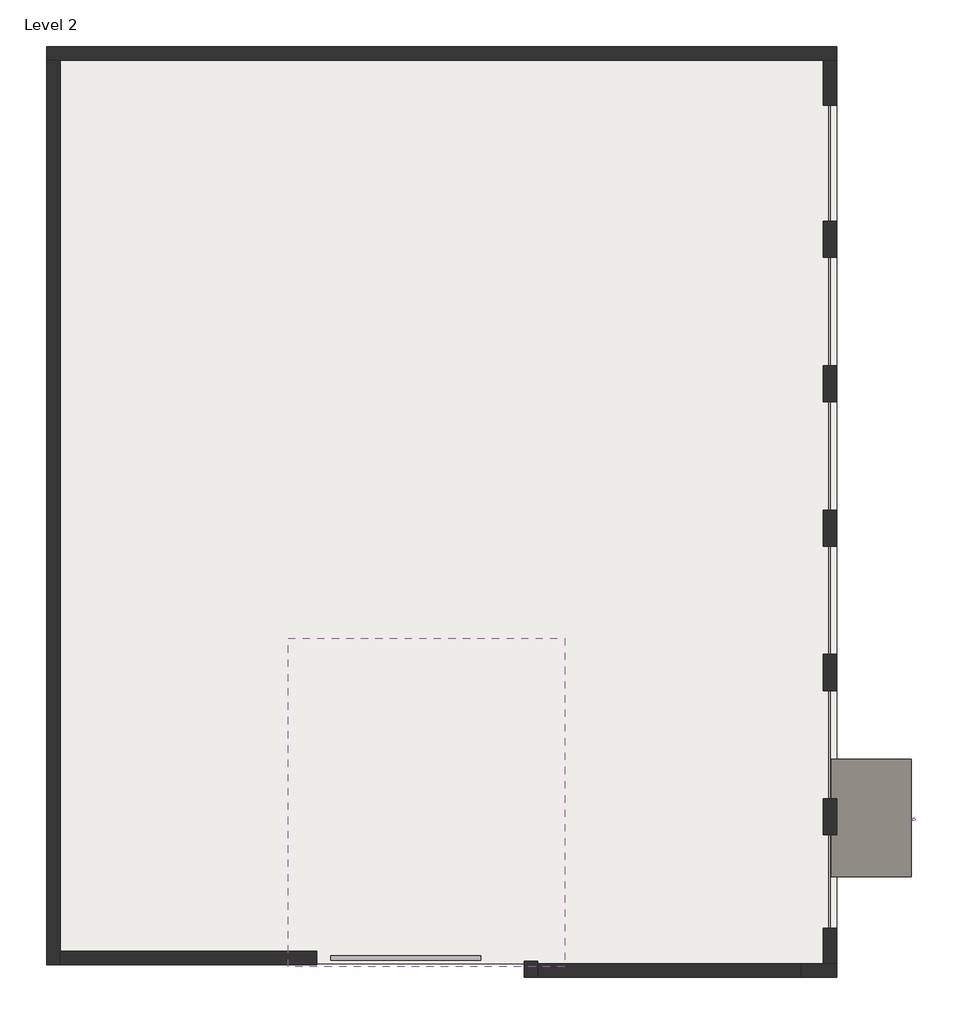
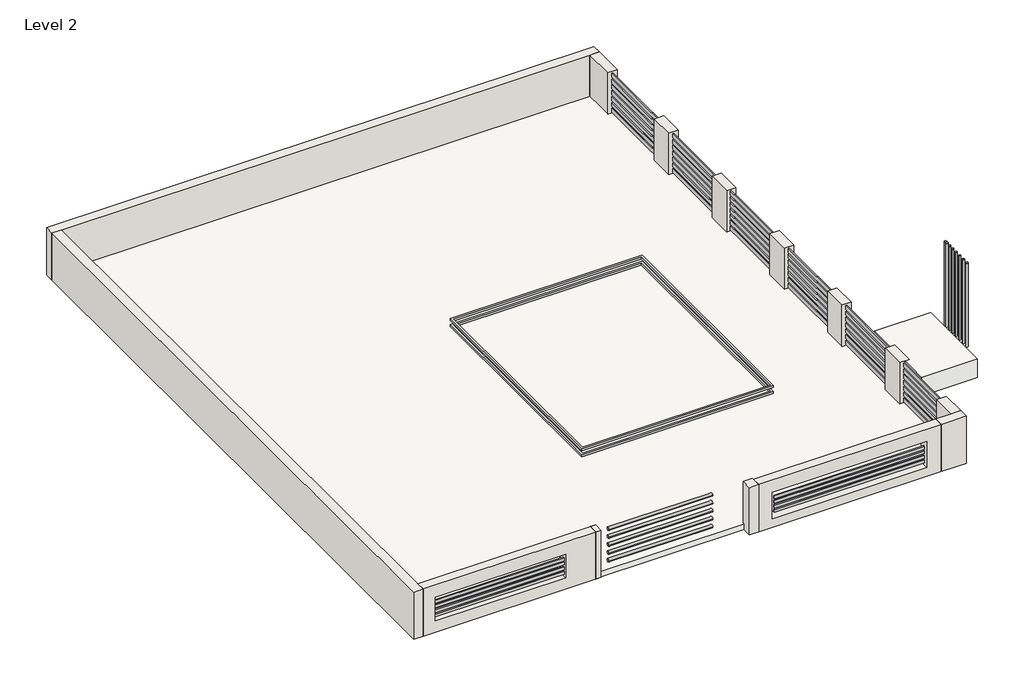
# One storey: 15 walls, 6 proxies, 1 covering, 1 slab.
"""IFC4 building model written with IfcOpenShell, lengths in millimetres."""

from ifc_helpers import new_model, si_unit, frame, origin, place, context, project, spatial, polyline, outline, extrude, faceted_brep, transform, mapped, element, save
from components import generic_models_12_generic_models_12_e0019dea, generic_models_2_generic_models_2_a69240e3, generic_models_3_generic_models_3_31b21ce6, generic_models_8_generic_models_8_cbadd6cc, railing_ms_1_railing_ms_1_2379e55e, railing_ms_2_railing_ms_1_4ed16cdf

model = new_model("IFC4")

# Units and contexts
model_context = context("Model", 3, world=origin())
ifc_project = project(units=[si_unit("LENGTHUNIT", "METRE", prefix="MILLI")], contexts=[model_context])

# Site, building, storey
site = spatial("IfcSite", under=ifc_project)
building = spatial("IfcBuilding", under=site)
storey = spatial("IfcBuildingStorey", under=building, Name="Level 2", Elevation=6705.6)

# Proxies
placement = place(None, origin())
generic_models_12_generic_models_12_shape = generic_models_12_generic_models_12_e0019dea(model_context)
element("IfcBuildingElementProxy", 1, Name="Generic Models 12 : Generic Models 12", ObjectType="Generic Models 12 : Generic Models 12", at=placement, inside=storey, context=model_context, shape_type="MappedRepresentation", body=[
    mapped(generic_models_12_generic_models_12_shape, transform((0.0, 0.0, 0.0), x_axis=(1.0, 0.0, 0.0), y_axis=(0.0, 1.0, 0.0), z_axis=(0.0, 0.0, 1.0))),
])
generic_models_2_generic_models_2_shape = generic_models_2_generic_models_2_a69240e3(model_context)
element("IfcBuildingElementProxy", 2, Name="Generic Models 2 : Generic Models 2", ObjectType="Generic Models 2 : Generic Models 2", at=placement, inside=storey, context=model_context, shape_type="MappedRepresentation", body=[
    mapped(generic_models_2_generic_models_2_shape, transform((0.0, 0.0, 0.0), x_axis=(1.0, 0.0, 0.0), y_axis=(0.0, 1.0, 0.0), z_axis=(0.0, 0.0, 1.0))),
])
generic_models_3_generic_models_3_shape = generic_models_3_generic_models_3_31b21ce6(model_context)
element("IfcBuildingElementProxy", 3, Name="Generic Models 3 : Generic Models 3", ObjectType="Generic Models 3 : Generic Models 3", at=placement, inside=storey, context=model_context, shape_type="MappedRepresentation", body=[
    mapped(generic_models_3_generic_models_3_shape, transform((0.0, 0.0, 0.0), x_axis=(1.0, 0.0, 0.0), y_axis=(0.0, 1.0, 0.0), z_axis=(0.0, 0.0, 1.0))),
])
generic_models_8_generic_models_8_shape = generic_models_8_generic_models_8_cbadd6cc(model_context)
element("IfcBuildingElementProxy", 4, Name="Generic Models 8 : Generic Models 8", ObjectType="Generic Models 8 : Generic Models 8", at=placement, inside=storey, context=model_context, shape_type="MappedRepresentation", body=[
    mapped(generic_models_8_generic_models_8_shape, transform((0.0, 0.0, 0.0), x_axis=(1.0, 0.0, 0.0), y_axis=(0.0, 1.0, 0.0), z_axis=(0.0, 0.0, 1.0))),
])
railing_ms_1_railing_ms_1_shape = railing_ms_1_railing_ms_1_2379e55e(model_context)
element("IfcBuildingElementProxy", 5, Name="railing ms 1 : railing ms 1", ObjectType="railing ms 1 : railing ms 1", at=placement, inside=storey, context=model_context, shape_type="MappedRepresentation", body=[
    mapped(railing_ms_1_railing_ms_1_shape, transform((0.0, 0.0, 0.0), x_axis=(1.0, 0.0, 0.0), y_axis=(0.0, 1.0, 0.0), z_axis=(0.0, 0.0, 1.0))),
])
railing_ms_2_railing_ms_1_shape = railing_ms_2_railing_ms_1_4ed16cdf(model_context)
element("IfcBuildingElementProxy", 6, Name="railing ms 2 : railing ms 1", ObjectType="railing ms 2 : railing ms 1", at=placement, inside=storey, context=model_context, shape_type="MappedRepresentation", body=[
    mapped(railing_ms_2_railing_ms_1_shape, transform((8178.1160753, -127.0, -19.7286522), x_axis=(1.0, 0.0, 0.0), y_axis=(0.0, 1.0, 0.0), z_axis=(0.0, 0.0, 1.0))),
])

# Covering
element("IfcCovering", 7, ObjectType="300mm_Generic 3", at=placement, inside=storey, context=model_context, shape_type="SweptSolid", body=[
    extrude(outline(polyline([(-19412.729089, -4479.5968048), (-19412.729089, 10900.1031952), (-6179.329089, 10900.1031952), (-6179.329089, -4593.8968048), (-6788.929089, -4593.8968048), (-11348.229089, -4593.8968048), (-11348.229089, -4479.5968048), (-19412.729089, -4479.5968048)])), frame((0.0, 0.0, 6705.6), z_axis=(0.0, 0.0, 1.0), x_axis=(1.0, 0.0, 0.0)), (0.0, 0.0, 1.0), 152.4),
])

# Slab
element("IfcSlab", 8, ObjectType="Floor-Grnd-Susp_65Scr-80Ins-100Blk-75PC", at=placement, inside=storey, context=model_context, shape_type="SweptSolid", body=[
    extrude(outline(polyline([(-4918.5966301, -1025.1968048), (-4918.5966301, -3006.3968048), (-6274.579089, -3006.3968048), (-6274.579089, -1025.1968048), (-4918.5966301, -1025.1968048)])), frame((0.0, 0.0, 7448.45), z_axis=(0.0, 0.0, 1.0), x_axis=(1.0, 0.0, 0.0)), (0.0, 0.0, 1.0), 470.0),
])

# Walls
element("IfcWall", 9, ObjectType="basic wall 2", at=placement, inside=storey, context=model_context, shape_type="Brep", body=[
    faceted_brep([(-6179.329089, 11014.4031952, 6705.6), (-19527.029089, 11014.4031952, 6705.6), (-19527.029089, 11014.4031952, 7924.8), (-6179.329089, 11014.4031952, 7924.8), (-6179.329089, 10785.8031952, 6705.6), (-6179.329089, 10785.8031952, 7924.8), (-6407.929089, 10785.8031952, 7924.8), (-19298.429089, 10785.8031952, 7924.8), (-19527.029089, 10785.8031952, 7924.8), (-19527.029089, 10785.8031952, 6705.6), (-19298.429089, 10785.8031952, 6705.6), (-6407.929089, 10785.8031952, 6705.6)], [[[0, 1, 2, 3]], [[4, 5, 6, 7, 8, 9, 10, 11]], [[1, 0, 4, 11, 10, 9]], [[3, 2, 8, 7, 6, 5]], [[2, 1, 9, 8]], [[0, 3, 5, 4]]]),
])
element("IfcWall", 10, ObjectType="basic wall 2", at=placement, inside=storey, context=model_context, shape_type="Brep", body=[
    faceted_brep([(-19527.029089, 10785.8031952, 6705.6), (-19527.029089, -4496.0724035, 6705.6), (-19527.029089, -4496.0724035, 7924.8), (-19527.029089, 10785.8031952, 7924.8), (-19298.429089, 10785.8031952, 6705.6), (-19298.429089, 10785.8031952, 7924.8), (-19298.429089, -4267.4724035, 7924.8), (-19298.429089, -4496.0724035, 7924.8), (-19298.429089, -4496.0724035, 6705.6), (-19298.429089, -4267.4724035, 6705.6)], [[[0, 1, 2, 3]], [[4, 5, 6, 7, 8, 9]], [[1, 0, 4, 9, 8]], [[3, 2, 7, 6, 5]], [[0, 3, 5, 4]], [[2, 1, 8, 7]]]),
])
element("IfcWall", 11, ObjectType="basic wall 2", at=placement, inside=storey, context=model_context, shape_type="SweptSolid", body=[
    extrude(outline(polyline([(6705.6, -19298.429089), (6705.6, -14961.379089), (7924.8, -14961.379089), (7924.8, -19298.429089), (6705.6, -19298.429089)]), holes=[polyline([(7605.6, -15821.923818), (6996.0, -15821.923818), (6996.0, -19004.329089), (7605.6, -19004.329089), (7605.6, -15821.923818)])]), frame((0.0, -4496.0724035, 0.0), z_axis=(0.0, 1.0, 0.0), x_axis=(0.0, 0.0, 1.0)), (0.0, 0.0, 1.0), 228.6),
])
element("IfcWall", 12, ObjectType="basic wall 2", at=placement, inside=storey, context=model_context, shape_type="SweptSolid", body=[
    extrude(outline(polyline([(6705.6, -11233.929089), (6705.6, -6788.929089), (7924.8, -6788.929089), (7924.8, -11233.929089), (6705.6, -11233.929089)]), holes=[polyline([(7605.6, -7141.2969384), (6930.6, -7141.2969384), (6930.6, -10904.329089), (7605.6, -10904.329089), (7605.6, -7141.2969384)])]), frame((0.0, -4708.1968048, 0.0), z_axis=(0.0, 1.0, 0.0), x_axis=(0.0, 0.0, 1.0)), (0.0, 0.0, 1.0), 228.6),
])
element("IfcWall", 13, ObjectType="basic wall 2", at=placement, inside=storey, context=model_context, shape_type="Brep", body=[
    faceted_brep([(-11233.929089, -4708.1968048, 6705.6), (-11233.929089, -4479.5968048, 6705.6), (-11233.929089, -4438.9224035, 6705.6), (-11233.929089, -4438.9224035, 7924.8), (-11233.929089, -4479.5968048, 7924.8), (-11233.929089, -4708.1968048, 7924.8), (-11462.529089, -4708.1968048, 6705.6), (-11462.529089, -4708.1968048, 7924.8), (-11462.529089, -4438.9224035, 7924.8), (-11462.529089, -4438.9224035, 6705.6)], [[[0, 1, 2, 3, 4, 5]], [[6, 7, 8, 9]], [[2, 1, 0, 6, 9]], [[5, 4, 3, 8, 7]], [[0, 5, 7, 6]], [[3, 2, 9, 8]]]),
])
element("IfcWall", 14, ObjectType="basic wall 2", at=placement, inside=storey, context=model_context, shape_type="Brep", body=[
    faceted_brep([(-6788.929089, -4708.1968048, 7924.8), (-6788.929089, -4708.1968048, 6705.6), (-6179.329089, -4708.1968048, 6705.6), (-6179.329089, -4708.1968048, 7924.8), (-6788.929089, -4479.5968048, 6705.6), (-6788.929089, -4479.5968048, 7924.8), (-6407.929089, -4479.5968048, 7924.8), (-6179.329089, -4479.5968048, 7924.8), (-6179.329089, -4479.5968048, 6705.6), (-6407.929089, -4479.5968048, 6705.6)], [[[0, 1, 2, 3]], [[4, 5, 6, 7, 8, 9]], [[2, 1, 4, 9, 8]], [[0, 3, 7, 6, 5]], [[0, 5, 4, 1]], [[3, 2, 8, 7]]]),
])
element("IfcWall", 15, ObjectType="basic wall 2", at=placement, inside=storey, context=model_context, shape_type="SweptSolid", body=[
    extrude(outline(polyline([(-15088.379089, -4267.4724035), (-14961.379089, -4267.4724035), (-14961.379089, -4496.0724035), (-15088.379089, -4496.0724035), (-15088.379089, -4267.4724035)])), frame((0.0, 0.0, 6705.6), z_axis=(0.0, 0.0, 1.0), x_axis=(1.0, 0.0, 0.0)), (0.0, 0.0, 1.0), 1219.2),
])
element("IfcWall", 16, ObjectType="basic wall 2", at=placement, inside=storey, context=model_context, shape_type="SweptSolid", body=[
    extrude(outline(polyline([(-6179.329089, -1691.9468048), (-6179.329089, -2301.5468048), (-6407.929089, -2301.5468048), (-6407.929089, -1691.9468048), (-6179.329089, -1691.9468048)])), frame((0.0, 0.0, 6705.6), z_axis=(0.0, 0.0, 1.0), x_axis=(1.0, 0.0, 0.0)), (0.0, 0.0, 1.0), 1219.2),
])
element("IfcWall", 17, ObjectType="basic wall 2", at=placement, inside=storey, context=model_context, shape_type="SweptSolid", body=[
    extrude(outline(polyline([(-6179.329089, 746.4531952), (-6179.329089, 136.8531952), (-6407.929089, 136.8531952), (-6407.929089, 746.4531952), (-6179.329089, 746.4531952)])), frame((0.0, 0.0, 6705.6), z_axis=(0.0, 0.0, 1.0), x_axis=(1.0, 0.0, 0.0)), (0.0, 0.0, 1.0), 1219.2),
])
element("IfcWall", 18, ObjectType="basic wall 2", at=placement, inside=storey, context=model_context, shape_type="SweptSolid", body=[
    extrude(outline(polyline([(-6179.329089, 3184.8531952), (-6179.329089, 2575.2531952), (-6407.929089, 2575.2531952), (-6407.929089, 3184.8531952), (-6179.329089, 3184.8531952)])), frame((0.0, 0.0, 6705.6), z_axis=(0.0, 0.0, 1.0), x_axis=(1.0, 0.0, 0.0)), (0.0, 0.0, 1.0), 1219.2),
])
element("IfcWall", 19, ObjectType="basic wall 2", at=placement, inside=storey, context=model_context, shape_type="SweptSolid", body=[
    extrude(outline(polyline([(-6179.329089, 5623.2531952), (-6179.329089, 5013.6531952), (-6407.929089, 5013.6531952), (-6407.929089, 5623.2531952), (-6179.329089, 5623.2531952)])), frame((0.0, 0.0, 6705.6), z_axis=(0.0, 0.0, 1.0), x_axis=(1.0, 0.0, 0.0)), (0.0, 0.0, 1.0), 1219.2),
])
element("IfcWall", 20, ObjectType="basic wall 2", at=placement, inside=storey, context=model_context, shape_type="SweptSolid", body=[
    extrude(outline(polyline([(-6179.329089, 8061.6531952), (-6179.329089, 7452.0531952), (-6407.929089, 7452.0531952), (-6407.929089, 8061.6531952), (-6179.329089, 8061.6531952)])), frame((0.0, 0.0, 6705.6), z_axis=(0.0, 0.0, 1.0), x_axis=(1.0, 0.0, 0.0)), (0.0, 0.0, 1.0), 1219.2),
])
element("IfcWall", 21, ObjectType="basic wall 2", at=placement, inside=storey, context=model_context, shape_type="SweptSolid", body=[
    extrude(outline(polyline([(-6179.329089, 10785.1419967), (-6179.329089, 10023.8031952), (-6407.929089, 10023.8031952), (-6407.929089, 10785.1419967), (-6179.329089, 10785.1419967)])), frame((0.0, 0.0, 6705.6), z_axis=(0.0, 0.0, 1.0), x_axis=(1.0, 0.0, 0.0)), (0.0, 0.0, 1.0), 1219.2),
])
element("IfcWall", 22, ObjectType="basic wall 2", at=placement, inside=storey, context=model_context, shape_type="SweptSolid", body=[
    extrude(outline(polyline([(-6179.329089, -3876.3468048), (-6179.329089, -4479.5968048), (-6407.929089, -4479.5968048), (-6407.929089, -3876.3468048), (-6179.329089, -3876.3468048)])), frame((0.0, 0.0, 6705.6), z_axis=(0.0, 0.0, 1.0), x_axis=(1.0, 0.0, 0.0)), (0.0, 0.0, 1.0), 1219.2),
])
element("IfcWall", 23, ObjectType="basic wall 2", at=placement, inside=storey, context=model_context, shape_type="SweptSolid", body=[
    extrude(outline(polyline([(-6179.329089, 10785.8031952), (-6179.329089, 10785.1419967), (-6407.929089, 10785.1419967), (-6407.929089, 10785.8031952), (-6179.329089, 10785.8031952)])), frame((0.0, 0.0, 6705.6), z_axis=(0.0, 0.0, 1.0), x_axis=(1.0, 0.0, 0.0)), (0.0, 0.0, 1.0), 1219.2),
])

save(model, "model.ifc")

# Revit data of these elements
# Type "300mm_Generic 3"
#   built-in parameter 1002203 = 1 (stored number, unit not read)
#   built-in parameter 1002202 = 1 (stored number, unit not read)
#   Layers, outside or top first: 0' - 6" "Air" (function 1)
# Type "Floor-Grnd-Susp_65Scr-80Ins-100Blk-75PC"
#   Keynote = "E60/130"
#   Function = 0
#   Layers, outside or top first: 0' - 2.55906" "Concrete, Sand/Cement Screed" (function 4); 0' - 0" "Vapor Retarder" (function 100); 0' - 3.14961" "Rigid insulation" (function 3); 0' - 5.90551" "Air" (function 3); 0' - 0" "Damp-proofing" (function 100); 0' - 3.93701" "Concrete Masonry, Floor Block" (function 1); 0' - 2.95276" "Concrete, Precast" (function 1)
# Type "basic wall 2"
#   Keynote = "F10"
#   Layers, outside or top first: 0' - 9" "Brick, Common" (function 1)
# Element 1 (IfcBuildingElementProxy, "Generic Models 12 : Generic Models 12")
#   Phase Created = New Construction
# Element 2 (IfcBuildingElementProxy, "Generic Models 2 : Generic Models 2")
#   Phase Created = New Construction
# Element 3 (IfcBuildingElementProxy, "Generic Models 3 : Generic Models 3")
#   Phase Created = New Construction
#   Materials on its faces: "Wood Planks"
# Element 4 (IfcBuildingElementProxy, "Generic Models 8 : Generic Models 8")
#   Phase Created = New Construction
#   Materials on its faces: "Damp-proofing"
# Element 5 (IfcBuildingElementProxy, "railing ms 1 : railing ms 1")
#   Phase Created = New Construction
# Element 6 (IfcBuildingElementProxy, "railing ms 2 : railing ms 1")
#   Phase Created = New Construction
# Element 7 (IfcCovering, "300mm_Generic 3")
#   Height Offset From Level = 0' - 0"
#   Phase Created = New Construction
#   Materials on its faces: "Air"
# Element 8 (IfcSlab, "Floor-Grnd-Susp_65Scr-80Ins-100Blk-75PC")
#   Height Offset From Level = 3' - 11 3/4"
#   Phase Created = New Construction
#   Materials on its faces: "Concrete, Precast", "Concrete, Sand/Cement Screed"
# Elements 9, 10, 11, 12, 13, 14, 15, 16, 17, 18, 19, 20, 21, 22, 23 (IfcWall, "basic wall 2")
#   Top Offset = 0' - 0"
#   Base Offset = 0' - 0"
#   Unconnected Height = 4' - 0"
#   wall height = 4' - 0"
#   Phase Created = New Construction
#   Base Constraint = Level 2
#   Materials on its faces: "Brick, Common"
# Materials
#   "Air": class "Gas", colour RGB 255 255 255, transparency 0, Description = "Air", Cost = 0
#   "Concrete, Sand/Cement Screed": class "Concrete", colour RGB 127 127 127, transparency 0, Description = "Concrete slab topping", Cost = 0
#   "Vapor Retarder": class "Generic", colour RGB 120 120 120, transparency 0, Description = "Polyethylene film membrane", Cost = 0
#   "Rigid insulation": class "Generic", colour RGB 127 127 127, transparency 0, Description = "Rigid foam insulation board", Cost = 0
#   "Damp-proofing": class "Generic", colour RGB 127 127 127, transparency 0, Description = "Damp-proofing", Cost = 0
#   "Concrete Masonry, Floor Block": class "Concrete", colour RGB 152 154 138, transparency 0, Description = "physical material", Cost = 0
#   "Concrete, Precast": class "Concrete", colour RGB 192 192 192, transparency 0, Description = "Precast concrete", Cost = 0
#   "Brick, Common": class "Masonry", colour RGB 170 100 105, transparency 0, Description = "Common brick", Cost = 0
#   "Wood Planks": class "Wood", colour RGB 129 72 39, transparency 0, Description = "Physical material.", Cost = 0
